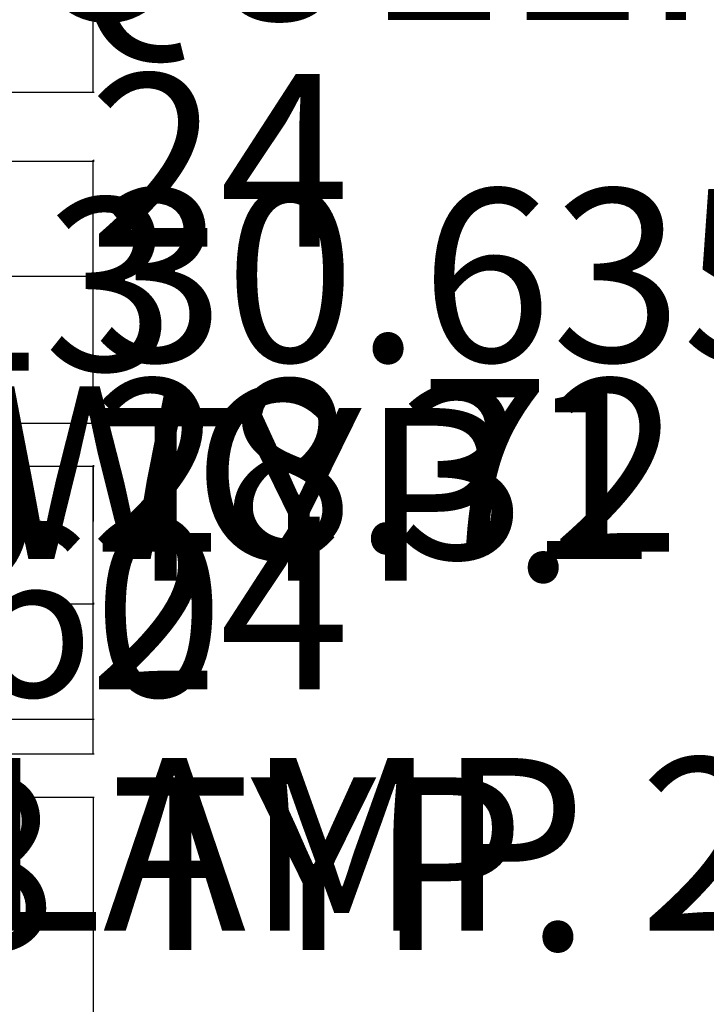
# Model space of a CAD drawing. Units: inches. Extents: x 1173 to 2157, y 515 to 1129.
# Tile 9 of 13: x 1681 to 1824, y 743 to 948. Entities that reach past the tile are written whole.
import ezdxf

# ---------------------------------------------------------------- set-up
doc = ezdxf.new("R2010")
doc.units = ezdxf.units.IN
doc.header["$MEASUREMENT"] = 0
doc.layers.add('A-ANNO-DIMS', color=2, linetype='Continuous', lineweight=18)
doc.styles.get("Standard").update_dxf_attribs({"font": 'arial.ttf'})
doc.dimstyles.get("Standard").update_dxf_attribs({"dimtxt": 36, "dimasz": 0.18, "dimexe": 0.18, "dimexo": 0.0625, "dimgap": 0.09, "dimtad": 0, "dimtih": 1, "dimtoh": 1, "dimdec": 0, "dimrnd": 72, "dimzin": 0, "dimdsep": 46, "dimlunit": 3, "dimtxsty": 'Standard', "dimcen": 2, "dimadec": 0, "dimazin": 0, "dimtfac": 1, "dimtdec": 0, "dimtofl": 0, "dimtmove": 0, "dimatfit": 3, "dimfxl": 1, "dimtolj": 1, "dimtzin": 0, "dimarcsym": 0})

# ---------------------------------------------------------------- blocks, each defined once
blk = doc.blocks.new('*D26')
at = {"layer": 'A-ANNO-DIMS', "color": 0, "lineweight": -2, "transparency": 16777216}
for p, q in [((1577.15, 654.34), (1577.15, 661.66)), ((1577.33, 661.48), (1624.97, 661.48)), ((1625.15, 654.34), (1625.15, 661.66)), ((1625.15, 661.48), (1625.33, 661.48))]:
    blk.add_line(p, q, dxfattribs=at)
at = {"layer": 'A-ANNO-DIMS', "color": 0, "transparency": 16777216}
for points in [[(1577.33, 661.51), (1577.33, 661.45), (1577.15, 661.48)], [(1624.97, 661.51), (1624.97, 661.45), (1625.15, 661.48)]]:
    blk.add_solid(points, dxfattribs=at)
at = {"layer": 'Defpoints', "color": 0, "transparency": 16777216}
for p in [(1625.15, 661.48), (1577.15, 654.28), (1625.15, 654.28)]:
    blk.add_point(p, dxfattribs=at)
at = {"layer": 'A-ANNO-DIMS', "color": 0, "transparency": 16777216, "insert": (1831.09, 661.48), "char_height": 36, "attachment_point": 5}
blk.add_mtext('\\A1;WINDOW 48 TYP.', dxfattribs=at)
blk = doc.blocks.new('*D28')
at = {"layer": 'A-ANNO-DIMS', "color": 0, "lineweight": -2, "transparency": 16777216}
for p, q in [((1581.66, 978.31), (1581.66, 966.19)), ((1661.66, 978.31), (1661.66, 966.19)), ((1581.84, 966.37), (1661.48, 966.37)), ((1661.66, 966.37), (1661.84, 966.37))]:
    blk.add_line(p, q, dxfattribs=at)
at = {"layer": 'A-ANNO-DIMS', "color": 0, "transparency": 16777216}
for points in [[(1581.84, 966.4), (1581.84, 966.34), (1581.66, 966.37)], [(1661.48, 966.4), (1661.48, 966.34), (1661.66, 966.37)]]:
    blk.add_solid(points, dxfattribs=at)
at = {"layer": 'Defpoints', "color": 0, "transparency": 16777216}
for p in [(1581.66, 978.37), (1661.66, 978.37), (1661.66, 966.37)]:
    blk.add_point(p, dxfattribs=at)
at = {"layer": 'A-ANNO-DIMS', "color": 0, "transparency": 16777216, "insert": (1904.61, 966.37), "char_height": 36, "attachment_point": 5}
blk.add_mtext('\\A1;QUEEN BED 80 TYP.', dxfattribs=at)
blk = doc.blocks.new('*D30')
at = {"layer": 'A-ANNO-DIMS', "color": 0, "lineweight": -2, "transparency": 16777216}
for p, q in [((1555.97, 736.03), (1563.78, 736.03)), ((1563.6, 735.85), (1563.6, 729.12)), ((1563.6, 684.97), (1563.6, 691.71)), ((1555.97, 684.79), (1563.78, 684.79))]:
    blk.add_line(p, q, dxfattribs=at)
at = {"layer": 'A-ANNO-DIMS', "color": 0, "transparency": 16777216}
for points in [[(1563.57, 735.85), (1563.63, 735.85), (1563.6, 736.03)], [(1563.57, 684.97), (1563.63, 684.97), (1563.6, 684.79)]]:
    blk.add_solid(points, dxfattribs=at)
at = {"layer": 'Defpoints', "color": 0, "transparency": 16777216}
for p in [(1555.91, 736.03), (1563.6, 736.03), (1555.91, 684.79)]:
    blk.add_point(p, dxfattribs=at)
at = {"layer": 'A-ANNO-DIMS', "color": 0, "transparency": 16777216, "insert": (1563.6, 710.41), "char_height": 36, "attachment_point": 5}
blk.add_mtext('\\A1;DESK 51 TYP.', dxfattribs=at)
blk = doc.blocks.new('*D32')
at = {"layer": 'A-ANNO-DIMS', "color": 0, "lineweight": -2, "transparency": 16777216}
for p, q in [((1632.82, 772.28), (1632.82, 776.62)), ((1633, 776.44), (1660.73, 776.44)), ((1660.91, 772.28), (1660.91, 776.62)), ((1660.91, 776.44), (1661.09, 776.44))]:
    blk.add_line(p, q, dxfattribs=at)
at = {"layer": 'A-ANNO-DIMS', "color": 0, "transparency": 16777216}
for points in [[(1633, 776.47), (1633, 776.41), (1632.82, 776.44)], [(1660.73, 776.47), (1660.73, 776.41), (1660.91, 776.44)]]:
    blk.add_solid(points, dxfattribs=at)
at = {"layer": 'Defpoints', "color": 0, "transparency": 16777216}
for p in [(1660.91, 776.44), (1632.82, 772.22), (1660.91, 772.22)]:
    blk.add_point(p, dxfattribs=at)
at = {"layer": 'A-ANNO-DIMS', "color": 0, "transparency": 16777216, "insert": (1823.46, 776.44), "char_height": 36, "attachment_point": 5}
blk.add_mtext('\\A1;LAMP 28 TYP.', dxfattribs=at)
blk = doc.blocks.new('*D33')
at = {"layer": 'A-ANNO-DIMS', "color": 0, "lineweight": -2, "transparency": 16777216}
for p, q in [((1632.75, 772.22), (1628.42, 772.22)), ((1628.6, 772.22), (1628.6, 772.4)), ((1628.6, 772.4), (1628.78, 772.4)), ((1628.6, 744.31), (1628.6, 772.04)), ((1632.75, 744.13), (1628.42, 744.13))]:
    blk.add_line(p, q, dxfattribs=at)
at = {"layer": 'A-ANNO-DIMS', "color": 0, "transparency": 16777216}
for points in [[(1628.57, 772.04), (1628.63, 772.04), (1628.6, 772.22)], [(1628.57, 744.31), (1628.63, 744.31), (1628.6, 744.13)]]:
    blk.add_solid(points, dxfattribs=at)
at = {"layer": 'Defpoints', "color": 0, "transparency": 16777216}
for p in [(1628.6, 772.22), (1632.82, 772.22), (1632.82, 744.13)]:
    blk.add_point(p, dxfattribs=at)
at = {"layer": 'A-ANNO-DIMS', "color": 0, "transparency": 16777216, "insert": (1716.8, 772.4), "char_height": 36, "attachment_point": 5}
blk.add_mtext('\\A1;28 TYP.', dxfattribs=at)
blk = doc.blocks.new('*D34')
at = {"layer": 'A-ANNO-DIMS', "color": 0, "lineweight": -2, "transparency": 16777216}
for p, q in [((1631.9, 978.41), (1631.9, 982.97)), ((1632.08, 982.79), (1661.32, 982.79)), ((1661.5, 978.41), (1661.5, 982.97)), ((1661.5, 982.79), (1661.68, 982.79))]:
    blk.add_line(p, q, dxfattribs=at)
at = {"layer": 'A-ANNO-DIMS', "color": 0, "transparency": 16777216}
for points in [[(1632.08, 982.82), (1632.08, 982.76), (1631.9, 982.79)], [(1661.32, 982.82), (1661.32, 982.76), (1661.5, 982.79)]]:
    blk.add_solid(points, dxfattribs=at)
at = {"layer": 'Defpoints', "color": 0, "transparency": 16777216}
for p in [(1661.5, 982.79), (1631.9, 978.35), (1661.5, 978.35)]:
    blk.add_point(p, dxfattribs=at)
at = {"layer": 'A-ANNO-DIMS', "color": 0, "transparency": 16777216, "insert": (1918.96, 982.79), "char_height": 36, "attachment_point": 5}
blk.add_mtext('\\A1;NIGHTSTAND 30 TYP.', dxfattribs=at)
blk = doc.blocks.new('*D35')
at = {"layer": 'A-ANNO-DIMS', "color": 0, "lineweight": -2, "transparency": 16777216}
for p, q in [((1631.84, 978.35), (1627.28, 978.35)), ((1627.46, 978.35), (1627.46, 978.53)), ((1627.46, 978.53), (1627.64, 978.53)), ((1627.46, 949.05), (1627.46, 978.17)), ((1631.84, 948.87), (1627.28, 948.87))]:
    blk.add_line(p, q, dxfattribs=at)
at = {"layer": 'A-ANNO-DIMS', "color": 0, "transparency": 16777216}
for points in [[(1627.43, 978.17), (1627.49, 978.17), (1627.46, 978.35)], [(1627.43, 949.05), (1627.49, 949.05), (1627.46, 948.87)]]:
    blk.add_solid(points, dxfattribs=at)
at = {"layer": 'Defpoints', "color": 0, "transparency": 16777216}
for p in [(1627.46, 978.35), (1631.9, 978.35), (1631.9, 948.87)]:
    blk.add_point(p, dxfattribs=at)
at = {"layer": 'A-ANNO-DIMS', "color": 0, "transparency": 16777216, "insert": (1715.66, 978.53), "char_height": 36, "attachment_point": 5}
blk.add_mtext('\\A1;29 TYP.', dxfattribs=at)
blk = doc.blocks.new('*D44')
at = {"layer": 'A-ANNO-DIMS', "color": 0, "lineweight": -2, "transparency": 16777216}
for p, q in [((1630.26, 849.3), (1630.26, 854.13)), ((1630.44, 853.95), (1661.48, 853.95)), ((1661.66, 849.3), (1661.66, 854.13)), ((1661.66, 853.95), (1661.84, 853.95))]:
    blk.add_line(p, q, dxfattribs=at)
at = {"layer": 'A-ANNO-DIMS', "color": 0, "transparency": 16777216}
for points in [[(1630.44, 853.98), (1630.44, 853.92), (1630.26, 853.95)], [(1661.48, 853.98), (1661.48, 853.92), (1661.66, 853.95)]]:
    blk.add_solid(points, dxfattribs=at)
at = {"layer": 'Defpoints', "color": 0, "transparency": 16777216}
for p in [(1661.66, 853.95), (1630.26, 849.24), (1661.66, 849.24)]:
    blk.add_point(p, dxfattribs=at)
at = {"layer": 'A-ANNO-DIMS', "color": 0, "transparency": 16777216, "insert": (1799.17, 853.95), "char_height": 36, "attachment_point": 5}
blk.add_mtext('\\A1;WC 31 TYP.', dxfattribs=at)
blk = doc.blocks.new('*D45')
at = {"layer": 'A-ANNO-DIMS', "color": 0, "lineweight": -2, "transparency": 16777216}
for p, q in [((1630.2, 849.24), (1625.37, 849.24)), ((1625.55, 849.24), (1625.55, 849.42)), ((1625.55, 849.42), (1625.73, 849.42)), ((1625.55, 829.46), (1625.55, 849.06)), ((1630.2, 829.28), (1625.37, 829.28))]:
    blk.add_line(p, q, dxfattribs=at)
at = {"layer": 'A-ANNO-DIMS', "color": 0, "transparency": 16777216}
for points in [[(1625.52, 849.06), (1625.58, 849.06), (1625.55, 849.24)], [(1625.52, 829.46), (1625.58, 829.46), (1625.55, 829.28)]]:
    blk.add_solid(points, dxfattribs=at)
at = {"layer": 'Defpoints', "color": 0, "transparency": 16777216}
for p in [(1625.55, 849.24), (1630.26, 849.24), (1630.26, 829.28)]:
    blk.add_point(p, dxfattribs=at)
at = {"layer": 'A-ANNO-DIMS', "color": 0, "transparency": 16777216, "insert": (1713.74, 849.42), "char_height": 36, "attachment_point": 5}
blk.add_mtext('\\A1;20 TYP.', dxfattribs=at)
blk = doc.blocks.new('*D47')
at = {"layer": 'A-ANNO-DIMS', "color": 0, "lineweight": -2, "transparency": 16777216}
for p, q in [((1648.26, 896), (1648.18, 893.48)), ((1661.4, 895.58), (1661.32, 893.06)), ((1648.36, 893.65), (1661.15, 893.24)), ((1661.33, 893.24), (1661.51, 893.23))]:
    blk.add_line(p, q, dxfattribs=at)
at = {"layer": 'A-ANNO-DIMS', "color": 0, "transparency": 16777216}
for points in [[(1648.37, 893.68), (1648.36, 893.62), (1648.18, 893.66)], [(1661.15, 893.27), (1661.15, 893.21), (1661.33, 893.24)]]:
    blk.add_solid(points, dxfattribs=at)
at = {"layer": 'Defpoints', "color": 0, "transparency": 16777216}
for p in [(1648.26, 896.06), (1661.4, 895.64), (1661.33, 893.24)]:
    blk.add_point(p, dxfattribs=at)
at = {"layer": 'A-ANNO-DIMS', "color": 0, "transparency": 16777216, "insert": (1685.69, 893.23), "char_height": 36, "attachment_point": 5}
blk.add_mtext('\\A1;13', dxfattribs=at)
blk = doc.blocks.new('*D84')
at = {"layer": 'A-ANNO-DIMS', "color": 0, "lineweight": -2, "transparency": 16777216}
for p, q in [((1661.73, 786.28), (1696.15, 786.28)), ((1695.97, 786.1), (1695.97, 738.76)), ((1695.97, 654.46), (1695.97, 701.8)), ((1661.73, 654.28), (1696.15, 654.28))]:
    blk.add_line(p, q, dxfattribs=at)
at = {"layer": 'A-ANNO-DIMS', "color": 0, "transparency": 16777216}
for points in [[(1695.94, 786.1), (1696, 786.1), (1695.97, 786.28)], [(1695.94, 654.46), (1696, 654.46), (1695.97, 654.28)]]:
    blk.add_solid(points, dxfattribs=at)
at = {"layer": 'Defpoints', "color": 0, "transparency": 16777216}
for p in [(1661.66, 786.28), (1661.66, 654.28), (1695.97, 654.28)]:
    blk.add_point(p, dxfattribs=at)
at = {"layer": 'A-ANNO-DIMS', "color": 0, "transparency": 16777216, "insert": (1695.97, 720.28), "char_height": 36, "attachment_point": 5}
blk.add_mtext('\\A1;132', dxfattribs=at)
blk = doc.blocks.new('*D90')
at = {"layer": 'A-ANNO-DIMS', "color": 0, "lineweight": -2, "transparency": 16777216}
for p, q in [((1661.73, 1044.28), (1696.15, 1044.28)), ((1695.97, 1044.1), (1695.97, 1006.94)), ((1695.97, 933.46), (1695.97, 970.62)), ((1625.73, 933.28), (1696.15, 933.28))]:
    blk.add_line(p, q, dxfattribs=at)
at = {"layer": 'A-ANNO-DIMS', "color": 0, "transparency": 16777216}
for points in [[(1695.94, 1044.1), (1696, 1044.1), (1695.97, 1044.28)], [(1695.94, 933.46), (1696, 933.46), (1695.97, 933.28)]]:
    blk.add_solid(points, dxfattribs=at)
at = {"layer": 'Defpoints', "color": 0, "transparency": 16777216}
for p in [(1661.66, 1044.28), (1625.66, 933.28), (1695.97, 933.28)]:
    blk.add_point(p, dxfattribs=at)
at = {"layer": 'A-ANNO-DIMS', "color": 0, "transparency": 16777216, "insert": (1695.97, 988.78), "char_height": 36, "attachment_point": 5}
blk.add_mtext('\\A1;111', dxfattribs=at)
blk = doc.blocks.new('*D96')
at = {"layer": 'A-ANNO-DIMS', "color": 0, "lineweight": -2, "transparency": 16777216}
for p, q in [((1661.73, 855.28), (1696.15, 855.28)), ((1695.97, 855.1), (1695.97, 843.75)), ((1695.97, 795.46), (1695.97, 806.81)), ((1661.73, 795.28), (1696.15, 795.28))]:
    blk.add_line(p, q, dxfattribs=at)
at = {"layer": 'A-ANNO-DIMS', "color": 0, "transparency": 16777216}
for points in [[(1695.94, 855.1), (1696, 855.1), (1695.97, 855.28)], [(1695.94, 795.46), (1696, 795.46), (1695.97, 795.28)]]:
    blk.add_solid(points, dxfattribs=at)
at = {"layer": 'Defpoints', "color": 0, "transparency": 16777216}
for p in [(1661.66, 855.28), (1695.97, 855.28), (1661.66, 795.28)]:
    blk.add_point(p, dxfattribs=at)
at = {"layer": 'A-ANNO-DIMS', "color": 0, "transparency": 16777216, "insert": (1695.97, 825.28), "char_height": 36, "attachment_point": 5}
blk.add_mtext('\\A1;60', dxfattribs=at)
blk = doc.blocks.new('*D98')
at = {"layer": 'A-ANNO-DIMS', "color": 0, "lineweight": -2, "transparency": 16777216}
for p, q in [((1625.66, 924.34), (1625.66, 1078.79)), ((1625.84, 1078.61), (1661.48, 1078.61)), ((1661.66, 924.34), (1661.66, 1078.79)), ((1661.66, 1078.61), (1661.84, 1078.61))]:
    blk.add_line(p, q, dxfattribs=at)
at = {"layer": 'A-ANNO-DIMS', "color": 0, "transparency": 16777216}
for points in [[(1625.84, 1078.64), (1625.84, 1078.58), (1625.66, 1078.61)], [(1661.48, 1078.64), (1661.48, 1078.58), (1661.66, 1078.61)]]:
    blk.add_solid(points, dxfattribs=at)
at = {"layer": 'Defpoints', "color": 0, "transparency": 16777216}
for p in [(1661.66, 1078.61), (1625.66, 924.28), (1661.66, 924.28)]:
    blk.add_point(p, dxfattribs=at)
at = {"layer": 'A-ANNO-DIMS', "color": 0, "transparency": 16777216, "insert": (1687.69, 1078.61), "char_height": 36, "attachment_point": 5}
blk.add_mtext('\\A1;36', dxfattribs=at)
blk = doc.blocks.new('*D99')
at = {"layer": 'A-ANNO-DIMS', "color": 0, "lineweight": -2, "transparency": 16777216}
for p, q in [((1670.73, 918.92), (1696.15, 918.92)), ((1695.97, 918.92), (1695.97, 919.1)), ((1695.97, 919.1), (1696.15, 919.1)), ((1695.97, 895.1), (1695.97, 918.74)), ((1670.73, 894.92), (1696.15, 894.92))]:
    blk.add_line(p, q, dxfattribs=at)
at = {"layer": 'A-ANNO-DIMS', "color": 0, "transparency": 16777216}
for points in [[(1695.94, 918.74), (1696, 918.74), (1695.97, 918.92)], [(1695.94, 895.1), (1696, 895.1), (1695.97, 894.92)]]:
    blk.add_solid(points, dxfattribs=at)
at = {"layer": 'Defpoints', "color": 0, "transparency": 16777216}
for p in [(1670.66, 918.92), (1695.97, 918.92), (1670.66, 894.92)]:
    blk.add_point(p, dxfattribs=at)
at = {"layer": 'A-ANNO-DIMS', "color": 0, "transparency": 16777216, "insert": (1722.25, 919.1), "char_height": 36, "attachment_point": 5}
blk.add_mtext('\\A1;24', dxfattribs=at)
blk = doc.blocks.new('*D100')
at = {"layer": 'A-ANNO-DIMS', "color": 0, "lineweight": -2, "transparency": 16777216}
for p, q in [((1661.73, 894.92), (1696.15, 894.92)), ((1695.97, 894.92), (1695.97, 895.1)), ((1695.97, 895.1), (1696.15, 895.1)), ((1695.97, 864.46), (1695.97, 894.74)), ((1661.73, 864.28), (1696.15, 864.28))]:
    blk.add_line(p, q, dxfattribs=at)
at = {"layer": 'A-ANNO-DIMS', "color": 0, "transparency": 16777216}
for points in [[(1695.94, 894.74), (1696, 894.74), (1695.97, 894.92)], [(1695.94, 864.46), (1696, 864.46), (1695.97, 864.28)]]:
    blk.add_solid(points, dxfattribs=at)
at = {"layer": 'Defpoints', "color": 0, "transparency": 16777216}
for p in [(1661.66, 894.92), (1695.97, 894.92), (1661.66, 864.28)]:
    blk.add_point(p, dxfattribs=at)
at = {"layer": 'A-ANNO-DIMS', "color": 0, "transparency": 16777216, "insert": (1771.08, 895.1), "char_height": 36, "attachment_point": 5}
blk.add_mtext('\\A1;30.635', dxfattribs=at)
blk = doc.blocks.new('*D101')
at = {"layer": 'A-ANNO-DIMS', "color": 0, "lineweight": -2, "transparency": 16777216}
for p, q in [((1670.73, 826.56), (1696.15, 826.56)), ((1695.97, 826.56), (1695.97, 826.74)), ((1695.97, 826.74), (1696.15, 826.74)), ((1695.97, 802.74), (1695.97, 826.38)), ((1670.73, 802.56), (1696.15, 802.56))]:
    blk.add_line(p, q, dxfattribs=at)
at = {"layer": 'A-ANNO-DIMS', "color": 0, "transparency": 16777216}
for points in [[(1695.94, 826.38), (1696, 826.38), (1695.97, 826.56)], [(1695.94, 802.74), (1696, 802.74), (1695.97, 802.56)]]:
    blk.add_solid(points, dxfattribs=at)
at = {"layer": 'Defpoints', "color": 0, "transparency": 16777216}
for p in [(1670.66, 826.56), (1695.97, 826.56), (1670.66, 802.56)]:
    blk.add_point(p, dxfattribs=at)
at = {"layer": 'A-ANNO-DIMS', "color": 0, "transparency": 16777216, "insert": (1722.25, 826.74), "char_height": 36, "attachment_point": 5}
blk.add_mtext('\\A1;24', dxfattribs=at)
blk = doc.blocks.new('*D102')
at = {"layer": 'A-ANNO-DIMS', "color": 0, "lineweight": -2, "transparency": 16777216}
for p, q in [((1661.73, 855.28), (1696.15, 855.28)), ((1695.97, 855.28), (1695.97, 855.46)), ((1695.97, 855.46), (1696.15, 855.46)), ((1695.97, 826.74), (1695.97, 855.1)), ((1670.73, 826.56), (1696.15, 826.56))]:
    blk.add_line(p, q, dxfattribs=at)
at = {"layer": 'A-ANNO-DIMS', "color": 0, "transparency": 16777216}
for points in [[(1695.94, 855.1), (1696, 855.1), (1695.97, 855.28)], [(1695.94, 826.74), (1696, 826.74), (1695.97, 826.56)]]:
    blk.add_solid(points, dxfattribs=at)
at = {"layer": 'Defpoints', "color": 0, "transparency": 16777216}
for p in [(1661.66, 855.28), (1695.97, 855.28), (1670.66, 826.56)]:
    blk.add_point(p, dxfattribs=at)
at = {"layer": 'A-ANNO-DIMS', "color": 0, "transparency": 16777216, "insert": (1757.1, 855.46), "char_height": 36, "attachment_point": 5}
blk.add_mtext('\\A1;28.72', dxfattribs=at)

msp = doc.modelspace()

# ---------------------------------------------------------------- dimensions: what is measured, and where the dimension line sits
at = {"layer": 'A-ANNO-DIMS'}
dim = msp.add_linear_dim(base=(1661.6635, 1078.6127), p1=(1625.6635, 924.2805), p2=(1661.6635, 924.2805), dimstyle='Standard', override={"dimdec": 0, "dimlfac": 1, "dimrnd": 0, "dimzin": 0, "dimdsep": 46, "dimlunit": 2}, dxfattribs=at)
dim.commit()
dim.dimension.update_dxf_attribs({"geometry": '*D98', "text_midpoint": (1687.6933, 1078.6127)})
for base, p1, p2, text, picture, middle in [((1661.6635, 966.3712), (1581.6634, 978.3712), (1661.6635, 978.3712), 'QUEEN BED <> TYP.', '*D28', (1904.6142, 966.3712)), ((1661.5047, 982.7919), (1631.9047, 978.3519), (1661.5047, 978.3519), 'NIGHTSTAND <> TYP.', '*D34', (1918.9562, 982.7919)), ((1661.6635, 853.9514), (1630.2601, 849.2409), (1661.6635, 849.2409), 'WC <> TYP.', '*D44', (1799.1681, 853.9514)), ((1660.9104, 776.4354), (1632.8165, 772.2213), (1660.9104, 772.2213), 'LAMP <> TYP.', '*D32', (1823.4628, 776.4354)), ((1625.1498, 661.4805), (1577.1498, 654.2805), (1625.1498, 654.2805), 'WINDOW <> TYP.', '*D26', (1831.0938, 661.4805))]:
    dim = msp.add_linear_dim(base=base, p1=p1, p2=p2, text=text, dimstyle='Standard', override={"dimdec": 0, "dimlfac": 1, "dimrnd": 0, "dimzin": 0, "dimdsep": 46, "dimlunit": 2}, dxfattribs=at)
    dim.commit()
    dim.dimension.update_dxf_attribs({"geometry": picture, "text_midpoint": middle})
for base, p1, p2, angle, override, picture, middle in [((1695.966, 933.2805), (1661.6635, 1044.2805), (1625.6635, 933.2805), 90, {"dimdec": 0, "dimlfac": 1, "dimrnd": 0, "dimzin": 0, "dimdsep": 46, "dimlunit": 2}, '*D90', (1695.966, 988.7805)), ((1695.966, 918.9156), (1670.6635, 894.9156), (1670.6635, 918.9156), 90, {"dimdec": 0, "dimlfac": 1, "dimrnd": 0, "dimzin": 0, "dimdsep": 46, "dimlunit": 2}, '*D99', (1722.2537, 919.0956)), ((1695.966, 894.9156), (1661.6635, 864.2805), (1661.6635, 894.9156), 90, {"dimdec": 3, "dimlfac": 1, "dimrnd": 0, "dimzin": 0, "dimdsep": 46, "dimlunit": 2}, '*D100', (1771.0845, 895.0956)), ((1661.327, 893.2368), (1648.2623, 896.0638), (1661.4044, 895.6403), 358.15447, {"dimdec": 0, "dimlfac": 1, "dimrnd": 0, "dimzin": 0, "dimdsep": 46, "dimlunit": 2}, '*D47', (1685.6869, 893.231)), ((1695.966, 855.2805), (1670.6635, 826.5597), (1661.6635, 855.2805), 90, {"dimdec": 2, "dimlfac": 1, "dimrnd": 0, "dimzin": 0, "dimdsep": 46, "dimlunit": 2}, '*D102', (1757.0995, 855.4605)), ((1695.966, 855.2805), (1661.6635, 795.2805), (1661.6635, 855.2805), 90, {"dimdec": 0, "dimlfac": 1, "dimrnd": 0, "dimzin": 0, "dimdsep": 46, "dimlunit": 2}, '*D96', (1695.966, 825.2805)), ((1695.966, 826.5597), (1670.6635, 802.5597), (1670.6635, 826.5597), 90, {"dimdec": 0, "dimlfac": 1, "dimrnd": 0, "dimzin": 0, "dimdsep": 46, "dimlunit": 2}, '*D101', (1722.2537, 826.7397)), ((1695.966, 654.2805), (1661.6635, 786.2805), (1661.6635, 654.2805), 90, {"dimdec": 0, "dimlfac": 1, "dimrnd": 0, "dimzin": 0, "dimdsep": 46, "dimlunit": 2}, '*D84', (1695.966, 720.2805))]:
    dim = msp.add_linear_dim(base=base, p1=p1, p2=p2, angle=angle, dimstyle='Standard', override=override, dxfattribs=at)
    dim.commit()
    dim.dimension.update_dxf_attribs({"geometry": picture, "text_midpoint": middle})
for base, p1, p2, text, picture, middle in [((1627.4647, 978.3519), (1631.9047, 948.8672), (1631.9047, 978.3519), '<> TYP.', '*D35', (1715.6597, 978.5319)), ((1625.5496, 849.2409), (1630.2601, 829.2849), (1630.2601, 849.2409), '<> TYP.', '*D45', (1713.7446, 849.4209)), ((1628.6024, 772.2213), (1632.8165, 744.1274), (1632.8165, 772.2213), '<> TYP.', '*D33', (1716.7974, 772.4013)), ((1563.5964, 736.0322), (1555.9105, 684.7928), (1555.9105, 736.0322), 'DESK <> TYP.', '*D30', (1563.5964, 710.4125))]:
    dim = msp.add_linear_dim(base=base, p1=p1, p2=p2, angle=90, text=text, dimstyle='Standard', override={"dimdec": 0, "dimlfac": 1, "dimrnd": 0, "dimzin": 0, "dimdsep": 46, "dimlunit": 2}, dxfattribs=at)
    dim.commit()
    dim.dimension.update_dxf_attribs({"geometry": picture, "text_midpoint": middle})

doc.saveas('drawing.dxf')
